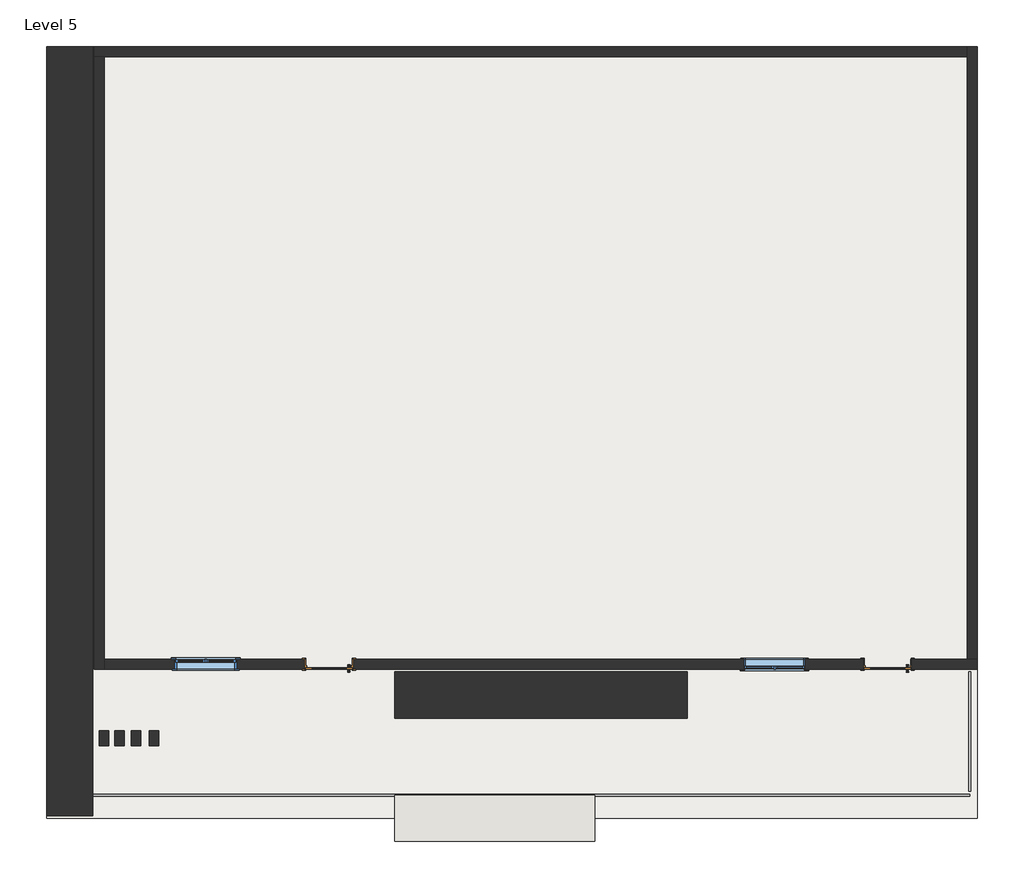
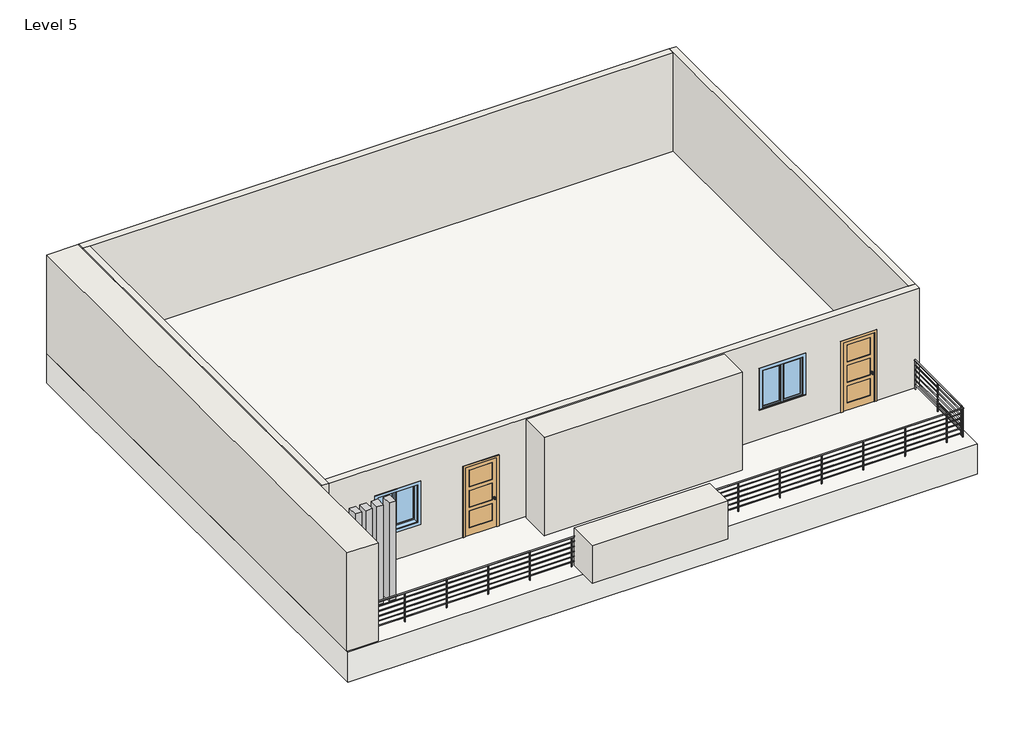
# One storey: 7 walls, 4 columns, 2 doors, 2 railings, 2 windows, 1 slab.
"""IFC4 building model written with IfcOpenShell, lengths in millimetres."""

from ifc_helpers import new_model, si_unit, point, frame, frame_2d, origin, place, context, project, spatial, polyline, circle_curve, trimmed, segment, composite_curve, outline, extrude, faceted_brep, transform, mapped, element, save
from components import wood_timber_column_8_x_12_7c9a4679, door_54d869bf, window_3a1167bf, window_0862ab64

model = new_model("IFC4")

# Units and contexts
model_context = context("Model", 3, world=origin())
ifc_project = project(units=[si_unit("LENGTHUNIT", "METRE", prefix="MILLI")], contexts=[model_context])

# Site, building, storey
site = spatial("IfcSite", under=ifc_project)
building = spatial("IfcBuilding", under=site)
storey = spatial("IfcBuildingStorey", under=building, Name="Level 5", Elevation=12192.0)

# Columns
placement = place(None, origin())
wood_timber_column_8_x_12_shape = wood_timber_column_8_x_12_7c9a4679(model_context)
element("IfcColumn", 1, ObjectType="Wood Timber Column : 8 x 12", at=placement, inside=storey, context=model_context, shape_type="MappedRepresentation", body=[
    mapped(wood_timber_column_8_x_12_shape, transform((-18270.7121948, 4590.8323495, 0.0), x_axis=(1.0, 0.0, 0.0), y_axis=(0.0, 1.0, 0.0), z_axis=(0.0, 0.0, 1.0))),
])
element("IfcColumn", 2, ObjectType="Wood Timber Column : 8 x 12", at=placement, inside=storey, context=model_context, shape_type="MappedRepresentation", body=[
    mapped(wood_timber_column_8_x_12_shape, transform((-18600.9121948, 4590.8323495, 0.0), x_axis=(1.0, 0.0, 0.0), y_axis=(0.0, 1.0, 0.0), z_axis=(0.0, 0.0, 1.0))),
])
element("IfcColumn", 3, ObjectType="Wood Timber Column : 8 x 12", at=placement, inside=storey, context=model_context, shape_type="MappedRepresentation", body=[
    mapped(wood_timber_column_8_x_12_shape, transform((-18905.7121948, 4590.8323495, 0.0), x_axis=(1.0, 0.0, 0.0), y_axis=(0.0, 1.0, 0.0), z_axis=(0.0, 0.0, 1.0))),
])
element("IfcColumn", 4, ObjectType="Wood Timber Column : 8 x 12", at=placement, inside=storey, context=model_context, shape_type="MappedRepresentation", body=[
    mapped(wood_timber_column_8_x_12_shape, transform((-17915.1121948, 4590.8323495, 0.0), x_axis=(1.0, 0.0, 0.0), y_axis=(0.0, 1.0, 0.0), z_axis=(0.0, 0.0, 1.0))),
])

# Doors
door_shape = door_54d869bf(model_context)
element("IfcDoor", 5, ObjectType="Door-Interior-Single-3_Panel_Vert-Wood : 36\" x 84\" 2", at=placement, inside=storey, context=model_context, shape_type="MappedRepresentation", body=[
    mapped(door_shape, transform((-3405.3621948, 6054.574368, 11845.2339631), x_axis=(-1.0, 0.0, 0.0), y_axis=(0.0, -1.0, 0.0), z_axis=(0.0, 0.0, 1.0))),
])
element("IfcDoor", 6, ObjectType="Door-Interior-Single-3_Panel_Vert-Wood : 36\" x 84\" 2", at=placement, inside=storey, context=model_context, shape_type="MappedRepresentation", body=[
    mapped(door_shape, transform((-14454.3621948, 6054.574368, 11845.2339631), x_axis=(-1.0, 0.0, 0.0), y_axis=(0.0, -1.0, 0.0), z_axis=(0.0, 0.0, 1.0))),
])

# Railings
element("IfcRailing", 7, ObjectType="Handrail - Pipe", at=placement, inside=storey, context=model_context, shape_type="SweptSolid", body=[
    extrude(outline(composite_curve([segment(trimmed(circle_curve(frame_2d((3466.949368, 12740.5839631)), 19.05), [point((3447.899368, 12740.5839631))], [point((3485.999368, 12740.5839631))], False, "CARTESIAN"), True, "CONTINUOUS"), segment(trimmed(circle_curve(frame_2d((3466.949368, 12740.5839631)), 19.05), [point((3485.999368, 12740.5839631))], [point((3447.899368, 12740.5839631))], False, "CARTESIAN"), True, "CONTINUOUS")], self_intersect=False)), frame((-19331.1621948, 0.0, 0.0), z_axis=(1.0, 0.0, 0.0), x_axis=(0.0, 1.0, 0.0)), (0.0, 0.0, 1.0), 17551.4),
    extrude(outline(composite_curve([segment(trimmed(circle_curve(frame_2d((3466.949368, 12594.5339631)), 12.7), [point((3479.649368, 12594.5339631))], [point((3454.249368, 12594.5339631))], False, "CARTESIAN"), True, "CONTINUOUS"), segment(trimmed(circle_curve(frame_2d((3466.949368, 12594.5339631)), 12.7), [point((3454.249368, 12594.5339631))], [point((3479.649368, 12594.5339631))], False, "CARTESIAN"), True, "CONTINUOUS")], self_intersect=False)), frame((-19331.1621948, 0.0, 0.0), z_axis=(1.0, 0.0, 0.0), x_axis=(0.0, 1.0, 0.0)), (0.0, 0.0, 1.0), 17551.4),
    extrude(outline(composite_curve([segment(trimmed(circle_curve(frame_2d((3466.949368, 12442.1339631)), 12.7), [point((3479.649368, 12442.1339631))], [point((3454.249368, 12442.1339631))], False, "CARTESIAN"), True, "CONTINUOUS"), segment(trimmed(circle_curve(frame_2d((3466.949368, 12442.1339631)), 12.7), [point((3454.249368, 12442.1339631))], [point((3479.649368, 12442.1339631))], False, "CARTESIAN"), True, "CONTINUOUS")], self_intersect=False)), frame((-19331.1621948, 0.0, 0.0), z_axis=(1.0, 0.0, 0.0), x_axis=(0.0, 1.0, 0.0)), (0.0, 0.0, 1.0), 17551.4),
    extrude(outline(composite_curve([segment(trimmed(circle_curve(frame_2d((3466.949368, 12289.7339631)), 12.7), [point((3479.649368, 12289.7339631))], [point((3454.249368, 12289.7339631))], False, "CARTESIAN"), True, "CONTINUOUS"), segment(trimmed(circle_curve(frame_2d((3466.949368, 12289.7339631)), 12.7), [point((3454.249368, 12289.7339631))], [point((3479.649368, 12289.7339631))], False, "CARTESIAN"), True, "CONTINUOUS")], self_intersect=False)), frame((-19331.1621948, 0.0, 0.0), z_axis=(1.0, 0.0, 0.0), x_axis=(0.0, 1.0, 0.0)), (0.0, 0.0, 1.0), 17551.4),
    extrude(outline(composite_curve([segment(trimmed(circle_curve(frame_2d((3466.949368, 12137.3339631)), 12.7), [point((3479.649368, 12137.3339631))], [point((3454.249368, 12137.3339631))], False, "CARTESIAN"), True, "CONTINUOUS"), segment(trimmed(circle_curve(frame_2d((3466.949368, 12137.3339631)), 12.7), [point((3454.249368, 12137.3339631))], [point((3479.649368, 12137.3339631))], False, "CARTESIAN"), True, "CONTINUOUS")], self_intersect=False)), frame((-19331.1621948, 0.0, 0.0), z_axis=(1.0, 0.0, 0.0), x_axis=(0.0, 1.0, 0.0)), (0.0, 0.0, 1.0), 17551.4),
    extrude(outline(composite_curve([segment(trimmed(circle_curve(frame_2d((3466.949368, 11984.9339631)), 12.7), [point((3479.649368, 11984.9339631))], [point((3454.249368, 11984.9339631))], False, "CARTESIAN"), True, "CONTINUOUS"), segment(trimmed(circle_curve(frame_2d((3466.949368, 11984.9339631)), 12.7), [point((3454.249368, 11984.9339631))], [point((3479.649368, 11984.9339631))], False, "CARTESIAN"), True, "CONTINUOUS")], self_intersect=False)), frame((-19331.1621948, 0.0, 0.0), z_axis=(1.0, 0.0, 0.0), x_axis=(0.0, 1.0, 0.0)), (0.0, 0.0, 1.0), 17551.4),
    extrude(outline(composite_curve([segment(trimmed(circle_curve(frame_2d((-2262.3621948, 3466.949368)), 12.7), [point((-2262.3621948, 3479.649368))], [point((-2262.3621948, 3454.249368))], False, "CARTESIAN"), True, "CONTINUOUS"), segment(trimmed(circle_curve(frame_2d((-2262.3621948, 3466.949368)), 12.7), [point((-2262.3621948, 3454.249368))], [point((-2262.3621948, 3479.649368))], False, "CARTESIAN"), True, "CONTINUOUS")], self_intersect=False)), frame((0.0, 0.0, 11845.2339631), z_axis=(0.0, 0.0, 1.0), x_axis=(1.0, 0.0, 0.0)), (0.0, 0.0, 1.0), 876.3),
    extrude(outline(composite_curve([segment(trimmed(circle_curve(frame_2d((-3481.5621948, 3466.949368)), 12.7), [point((-3481.5621948, 3479.649368))], [point((-3481.5621948, 3454.249368))], False, "CARTESIAN"), True, "CONTINUOUS"), segment(trimmed(circle_curve(frame_2d((-3481.5621948, 3466.949368)), 12.7), [point((-3481.5621948, 3454.249368))], [point((-3481.5621948, 3479.649368))], False, "CARTESIAN"), True, "CONTINUOUS")], self_intersect=False)), frame((0.0, 0.0, 11845.2339631), z_axis=(0.0, 0.0, 1.0), x_axis=(1.0, 0.0, 0.0)), (0.0, 0.0, 1.0), 876.3),
    extrude(outline(composite_curve([segment(trimmed(circle_curve(frame_2d((-4700.7621948, 3466.949368)), 12.7), [point((-4700.7621948, 3479.649368))], [point((-4700.7621948, 3454.249368))], False, "CARTESIAN"), True, "CONTINUOUS"), segment(trimmed(circle_curve(frame_2d((-4700.7621948, 3466.949368)), 12.7), [point((-4700.7621948, 3454.249368))], [point((-4700.7621948, 3479.649368))], False, "CARTESIAN"), True, "CONTINUOUS")], self_intersect=False)), frame((0.0, 0.0, 11845.2339631), z_axis=(0.0, 0.0, 1.0), x_axis=(1.0, 0.0, 0.0)), (0.0, 0.0, 1.0), 876.3),
    extrude(outline(composite_curve([segment(trimmed(circle_curve(frame_2d((-5919.9621948, 3466.949368)), 12.7), [point((-5919.9621948, 3479.649368))], [point((-5919.9621948, 3454.249368))], False, "CARTESIAN"), True, "CONTINUOUS"), segment(trimmed(circle_curve(frame_2d((-5919.9621948, 3466.949368)), 12.7), [point((-5919.9621948, 3454.249368))], [point((-5919.9621948, 3479.649368))], False, "CARTESIAN"), True, "CONTINUOUS")], self_intersect=False)), frame((0.0, 0.0, 11845.2339631), z_axis=(0.0, 0.0, 1.0), x_axis=(1.0, 0.0, 0.0)), (0.0, 0.0, 1.0), 876.3),
    extrude(outline(composite_curve([segment(trimmed(circle_curve(frame_2d((-7139.1621948, 3466.949368)), 12.7), [point((-7139.1621948, 3479.649368))], [point((-7139.1621948, 3454.249368))], False, "CARTESIAN"), True, "CONTINUOUS"), segment(trimmed(circle_curve(frame_2d((-7139.1621948, 3466.949368)), 12.7), [point((-7139.1621948, 3454.249368))], [point((-7139.1621948, 3479.649368))], False, "CARTESIAN"), True, "CONTINUOUS")], self_intersect=False)), frame((0.0, 0.0, 11845.2339631), z_axis=(0.0, 0.0, 1.0), x_axis=(1.0, 0.0, 0.0)), (0.0, 0.0, 1.0), 876.3),
    extrude(outline(composite_curve([segment(trimmed(circle_curve(frame_2d((-8358.3621948, 3466.949368)), 12.7), [point((-8358.3621948, 3479.649368))], [point((-8358.3621948, 3454.249368))], False, "CARTESIAN"), True, "CONTINUOUS"), segment(trimmed(circle_curve(frame_2d((-8358.3621948, 3466.949368)), 12.7), [point((-8358.3621948, 3454.249368))], [point((-8358.3621948, 3479.649368))], False, "CARTESIAN"), True, "CONTINUOUS")], self_intersect=False)), frame((0.0, 0.0, 11845.2339631), z_axis=(0.0, 0.0, 1.0), x_axis=(1.0, 0.0, 0.0)), (0.0, 0.0, 1.0), 876.3),
    extrude(outline(composite_curve([segment(trimmed(circle_curve(frame_2d((-9577.5621948, 3466.949368)), 12.7), [point((-9577.5621948, 3479.649368))], [point((-9577.5621948, 3454.249368))], False, "CARTESIAN"), True, "CONTINUOUS"), segment(trimmed(circle_curve(frame_2d((-9577.5621948, 3466.949368)), 12.7), [point((-9577.5621948, 3454.249368))], [point((-9577.5621948, 3479.649368))], False, "CARTESIAN"), True, "CONTINUOUS")], self_intersect=False)), frame((0.0, 0.0, 11845.2339631), z_axis=(0.0, 0.0, 1.0), x_axis=(1.0, 0.0, 0.0)), (0.0, 0.0, 1.0), 876.3),
    extrude(outline(composite_curve([segment(trimmed(circle_curve(frame_2d((-10796.7621948, 3466.949368)), 12.7), [point((-10796.7621948, 3479.649368))], [point((-10796.7621948, 3454.249368))], False, "CARTESIAN"), True, "CONTINUOUS"), segment(trimmed(circle_curve(frame_2d((-10796.7621948, 3466.949368)), 12.7), [point((-10796.7621948, 3454.249368))], [point((-10796.7621948, 3479.649368))], False, "CARTESIAN"), True, "CONTINUOUS")], self_intersect=False)), frame((0.0, 0.0, 11845.2339631), z_axis=(0.0, 0.0, 1.0), x_axis=(1.0, 0.0, 0.0)), (0.0, 0.0, 1.0), 876.3),
    extrude(outline(composite_curve([segment(trimmed(circle_curve(frame_2d((-12015.9621948, 3466.949368)), 12.7), [point((-12015.9621948, 3479.649368))], [point((-12015.9621948, 3454.249368))], False, "CARTESIAN"), True, "CONTINUOUS"), segment(trimmed(circle_curve(frame_2d((-12015.9621948, 3466.949368)), 12.7), [point((-12015.9621948, 3454.249368))], [point((-12015.9621948, 3479.649368))], False, "CARTESIAN"), True, "CONTINUOUS")], self_intersect=False)), frame((0.0, 0.0, 11845.2339631), z_axis=(0.0, 0.0, 1.0), x_axis=(1.0, 0.0, 0.0)), (0.0, 0.0, 1.0), 876.3),
    extrude(outline(composite_curve([segment(trimmed(circle_curve(frame_2d((-13235.1621948, 3466.949368)), 12.7), [point((-13235.1621948, 3479.649368))], [point((-13235.1621948, 3454.249368))], False, "CARTESIAN"), True, "CONTINUOUS"), segment(trimmed(circle_curve(frame_2d((-13235.1621948, 3466.949368)), 12.7), [point((-13235.1621948, 3454.249368))], [point((-13235.1621948, 3479.649368))], False, "CARTESIAN"), True, "CONTINUOUS")], self_intersect=False)), frame((0.0, 0.0, 11845.2339631), z_axis=(0.0, 0.0, 1.0), x_axis=(1.0, 0.0, 0.0)), (0.0, 0.0, 1.0), 876.3),
    extrude(outline(composite_curve([segment(trimmed(circle_curve(frame_2d((-14454.3621948, 3466.949368)), 12.7), [point((-14454.3621948, 3479.649368))], [point((-14454.3621948, 3454.249368))], False, "CARTESIAN"), True, "CONTINUOUS"), segment(trimmed(circle_curve(frame_2d((-14454.3621948, 3466.949368)), 12.7), [point((-14454.3621948, 3454.249368))], [point((-14454.3621948, 3479.649368))], False, "CARTESIAN"), True, "CONTINUOUS")], self_intersect=False)), frame((0.0, 0.0, 11845.2339631), z_axis=(0.0, 0.0, 1.0), x_axis=(1.0, 0.0, 0.0)), (0.0, 0.0, 1.0), 876.3),
    extrude(outline(composite_curve([segment(trimmed(circle_curve(frame_2d((-15673.5621948, 3466.949368)), 12.7), [point((-15673.5621948, 3479.649368))], [point((-15673.5621948, 3454.249368))], False, "CARTESIAN"), True, "CONTINUOUS"), segment(trimmed(circle_curve(frame_2d((-15673.5621948, 3466.949368)), 12.7), [point((-15673.5621948, 3454.249368))], [point((-15673.5621948, 3479.649368))], False, "CARTESIAN"), True, "CONTINUOUS")], self_intersect=False)), frame((0.0, 0.0, 11845.2339631), z_axis=(0.0, 0.0, 1.0), x_axis=(1.0, 0.0, 0.0)), (0.0, 0.0, 1.0), 876.3),
    extrude(outline(composite_curve([segment(trimmed(circle_curve(frame_2d((-16892.7621948, 3466.949368)), 12.7), [point((-16892.7621948, 3479.649368))], [point((-16892.7621948, 3454.249368))], False, "CARTESIAN"), True, "CONTINUOUS"), segment(trimmed(circle_curve(frame_2d((-16892.7621948, 3466.949368)), 12.7), [point((-16892.7621948, 3454.249368))], [point((-16892.7621948, 3479.649368))], False, "CARTESIAN"), True, "CONTINUOUS")], self_intersect=False)), frame((0.0, 0.0, 11845.2339631), z_axis=(0.0, 0.0, 1.0), x_axis=(1.0, 0.0, 0.0)), (0.0, 0.0, 1.0), 876.3),
    extrude(outline(composite_curve([segment(trimmed(circle_curve(frame_2d((-18111.9621948, 3466.949368)), 12.7), [point((-18111.9621948, 3479.649368))], [point((-18111.9621948, 3454.249368))], False, "CARTESIAN"), True, "CONTINUOUS"), segment(trimmed(circle_curve(frame_2d((-18111.9621948, 3466.949368)), 12.7), [point((-18111.9621948, 3454.249368))], [point((-18111.9621948, 3479.649368))], False, "CARTESIAN"), True, "CONTINUOUS")], self_intersect=False)), frame((0.0, 0.0, 11845.2339631), z_axis=(0.0, 0.0, 1.0), x_axis=(1.0, 0.0, 0.0)), (0.0, 0.0, 1.0), 876.3),
    extrude(outline(composite_curve([segment(trimmed(circle_curve(frame_2d((-1792.4621948, 3466.949368)), 12.7), [point((-1792.4621948, 3479.649368))], [point((-1792.4621948, 3454.249368))], False, "CARTESIAN"), True, "CONTINUOUS"), segment(trimmed(circle_curve(frame_2d((-1792.4621948, 3466.949368)), 12.7), [point((-1792.4621948, 3454.249368))], [point((-1792.4621948, 3479.649368))], False, "CARTESIAN"), True, "CONTINUOUS")], self_intersect=False)), frame((0.0, 0.0, 11845.2339631), z_axis=(0.0, 0.0, 1.0), x_axis=(1.0, 0.0, 0.0)), (0.0, 0.0, 1.0), 876.3),
    extrude(outline(composite_curve([segment(trimmed(circle_curve(frame_2d((-19318.4621948, 3466.949368)), 12.7), [point((-19318.4621948, 3479.649368))], [point((-19318.4621948, 3454.249368))], False, "CARTESIAN"), True, "CONTINUOUS"), segment(trimmed(circle_curve(frame_2d((-19318.4621948, 3466.949368)), 12.7), [point((-19318.4621948, 3454.249368))], [point((-19318.4621948, 3479.649368))], False, "CARTESIAN"), True, "CONTINUOUS")], self_intersect=False)), frame((0.0, 0.0, 11845.2339631), z_axis=(0.0, 0.0, 1.0), x_axis=(1.0, 0.0, 0.0)), (0.0, 0.0, 1.0), 876.3),
])
element("IfcRailing", 8, ObjectType="Handrail - Pipe", at=placement, inside=storey, context=model_context, shape_type="SweptSolid", body=[
    extrude(outline(composite_curve([segment(trimmed(circle_curve(frame_2d((12740.5839631, -1779.7621948)), 19.05), [point((12740.5839631, -1760.7121948))], [point((12740.5839631, -1798.8121948))], False, "CARTESIAN"), True, "CONTINUOUS"), segment(trimmed(circle_curve(frame_2d((12740.5839631, -1779.7621948)), 19.05), [point((12740.5839631, -1798.8121948))], [point((12740.5839631, -1760.7121948))], False, "CARTESIAN"), True, "CONTINUOUS")], self_intersect=False)), frame((0.0, 3543.149368, 0.0), z_axis=(0.0, 1.0, 0.0), x_axis=(0.0, 0.0, 1.0)), (0.0, 0.0, 1.0), 2362.2),
    extrude(outline(composite_curve([segment(trimmed(circle_curve(frame_2d((12594.5339631, -1779.7621948)), 12.7), [point((12594.5339631, -1792.4621948))], [point((12594.5339631, -1767.0621948))], False, "CARTESIAN"), True, "CONTINUOUS"), segment(trimmed(circle_curve(frame_2d((12594.5339631, -1779.7621948)), 12.7), [point((12594.5339631, -1767.0621948))], [point((12594.5339631, -1792.4621948))], False, "CARTESIAN"), True, "CONTINUOUS")], self_intersect=False)), frame((0.0, 3543.149368, 0.0), z_axis=(0.0, 1.0, 0.0), x_axis=(0.0, 0.0, 1.0)), (0.0, 0.0, 1.0), 2362.2),
    extrude(outline(composite_curve([segment(trimmed(circle_curve(frame_2d((12442.1339631, -1779.7621948)), 12.7), [point((12442.1339631, -1792.4621948))], [point((12442.1339631, -1767.0621948))], False, "CARTESIAN"), True, "CONTINUOUS"), segment(trimmed(circle_curve(frame_2d((12442.1339631, -1779.7621948)), 12.7), [point((12442.1339631, -1767.0621948))], [point((12442.1339631, -1792.4621948))], False, "CARTESIAN"), True, "CONTINUOUS")], self_intersect=False)), frame((0.0, 3543.149368, 0.0), z_axis=(0.0, 1.0, 0.0), x_axis=(0.0, 0.0, 1.0)), (0.0, 0.0, 1.0), 2362.2),
    extrude(outline(composite_curve([segment(trimmed(circle_curve(frame_2d((12289.7339631, -1779.7621948)), 12.7), [point((12289.7339631, -1792.4621948))], [point((12289.7339631, -1767.0621948))], False, "CARTESIAN"), True, "CONTINUOUS"), segment(trimmed(circle_curve(frame_2d((12289.7339631, -1779.7621948)), 12.7), [point((12289.7339631, -1767.0621948))], [point((12289.7339631, -1792.4621948))], False, "CARTESIAN"), True, "CONTINUOUS")], self_intersect=False)), frame((0.0, 3543.149368, 0.0), z_axis=(0.0, 1.0, 0.0), x_axis=(0.0, 0.0, 1.0)), (0.0, 0.0, 1.0), 2362.2),
    extrude(outline(composite_curve([segment(trimmed(circle_curve(frame_2d((12137.3339631, -1779.7621948)), 12.7), [point((12137.3339631, -1792.4621948))], [point((12137.3339631, -1767.0621948))], False, "CARTESIAN"), True, "CONTINUOUS"), segment(trimmed(circle_curve(frame_2d((12137.3339631, -1779.7621948)), 12.7), [point((12137.3339631, -1767.0621948))], [point((12137.3339631, -1792.4621948))], False, "CARTESIAN"), True, "CONTINUOUS")], self_intersect=False)), frame((0.0, 3543.149368, 0.0), z_axis=(0.0, 1.0, 0.0), x_axis=(0.0, 0.0, 1.0)), (0.0, 0.0, 1.0), 2362.2),
    extrude(outline(composite_curve([segment(trimmed(circle_curve(frame_2d((11984.9339631, -1779.7621948)), 12.7), [point((11984.9339631, -1792.4621948))], [point((11984.9339631, -1767.0621948))], False, "CARTESIAN"), True, "CONTINUOUS"), segment(trimmed(circle_curve(frame_2d((11984.9339631, -1779.7621948)), 12.7), [point((11984.9339631, -1767.0621948))], [point((11984.9339631, -1792.4621948))], False, "CARTESIAN"), True, "CONTINUOUS")], self_intersect=False)), frame((0.0, 3543.149368, 0.0), z_axis=(0.0, 1.0, 0.0), x_axis=(0.0, 0.0, 1.0)), (0.0, 0.0, 1.0), 2362.2),
    extrude(outline(composite_curve([segment(trimmed(circle_curve(frame_2d((-1779.7621948, 4762.349368)), 12.7), [point((-1792.4621948, 4762.349368))], [point((-1767.0621948, 4762.349368))], False, "CARTESIAN"), True, "CONTINUOUS"), segment(trimmed(circle_curve(frame_2d((-1779.7621948, 4762.349368)), 12.7), [point((-1767.0621948, 4762.349368))], [point((-1792.4621948, 4762.349368))], False, "CARTESIAN"), True, "CONTINUOUS")], self_intersect=False)), frame((0.0, 0.0, 11845.2339631), z_axis=(0.0, 0.0, 1.0), x_axis=(1.0, 0.0, 0.0)), (0.0, 0.0, 1.0), 876.3),
    extrude(outline(composite_curve([segment(trimmed(circle_curve(frame_2d((-1779.7621948, 5892.649368)), 12.7), [point((-1792.4621948, 5892.649368))], [point((-1767.0621948, 5892.649368))], False, "CARTESIAN"), True, "CONTINUOUS"), segment(trimmed(circle_curve(frame_2d((-1779.7621948, 5892.649368)), 12.7), [point((-1767.0621948, 5892.649368))], [point((-1792.4621948, 5892.649368))], False, "CARTESIAN"), True, "CONTINUOUS")], self_intersect=False)), frame((0.0, 0.0, 11845.2339631), z_axis=(0.0, 0.0, 1.0), x_axis=(1.0, 0.0, 0.0)), (0.0, 0.0, 1.0), 876.3),
    extrude(outline(composite_curve([segment(trimmed(circle_curve(frame_2d((-1779.7621948, 3555.849368)), 12.7), [point((-1792.4621948, 3555.849368))], [point((-1767.0621948, 3555.849368))], False, "CARTESIAN"), True, "CONTINUOUS"), segment(trimmed(circle_curve(frame_2d((-1779.7621948, 3555.849368)), 12.7), [point((-1767.0621948, 3555.849368))], [point((-1792.4621948, 3555.849368))], False, "CARTESIAN"), True, "CONTINUOUS")], self_intersect=False)), frame((0.0, 0.0, 11845.2339631), z_axis=(0.0, 0.0, 1.0), x_axis=(1.0, 0.0, 0.0)), (0.0, 0.0, 1.0), 876.3),
])

# Slab
element("IfcSlab", 9, ObjectType="Generic - 3'", at=placement, inside=storey, context=model_context, shape_type="SweptSolid", body=[
    extrude(outline(polyline([(-1627.3621948, 18275.149368), (-1627.3621948, 3009.749368), (-20042.3621948, 3009.749368), (-20042.3621948, 18275.149368), (-1627.3621948, 18275.149368)])), frame((0.0, 0.0, 10930.8339631), z_axis=(0.0, 0.0, 1.0), x_axis=(1.0, 0.0, 0.0)), (0.0, 0.0, 1.0), 914.4),
])

# Walls
element("IfcWall", 10, ObjectType="Generic - 3' 2", at=placement, inside=storey, context=model_context, shape_type="SweptSolid", body=[
    extrude(outline(polyline([(-7367.7621948, 4990.949368), (-13158.9621948, 4990.949368), (-13158.9621948, 5905.349368), (-7367.7621948, 5905.349368), (-7367.7621948, 4990.949368)])), frame((0.0, 0.0, 11845.2339631), z_axis=(0.0, 0.0, 1.0), x_axis=(1.0, 0.0, 0.0)), (0.0, 0.0, 1.0), 3048.0),
])
element("IfcWall", 11, ObjectType="Generic - 3' 4", at=placement, inside=storey, context=model_context, shape_type="SweptSolid", body=[
    extrude(outline(polyline([(-9196.5621948, 2552.549368), (-13158.9621948, 2552.549368), (-13158.9621948, 3466.949368), (-9196.5621948, 3466.949368), (-9196.5621948, 2552.549368)])), frame((0.0, 0.0, 11845.2339631), z_axis=(0.0, 0.0, 1.0), x_axis=(1.0, 0.0, 0.0)), (0.0, 0.0, 1.0), 1165.3811612),
])
element("IfcWall", 12, ObjectType="Generic - 3' 4", at=placement, inside=storey, context=model_context, shape_type="SweptSolid", body=[
    extrude(outline(polyline([(-20042.3621948, 3060.549368), (-20042.3621948, 18275.149368), (-19127.9621948, 18275.149368), (-19127.9621948, 3060.549368), (-20042.3621948, 3060.549368)])), frame((0.0, 0.0, 11845.2339631), z_axis=(0.0, 0.0, 1.0), x_axis=(1.0, 0.0, 0.0)), (0.0, 0.0, 1.0), 3048.0),
])
element("IfcWall", 13, ObjectType="Generic - 8\"", at=placement, inside=storey, context=model_context, shape_type="Brep", body=[
    faceted_brep([(-19102.5621948, 18071.949368, 11845.2339631), (-18899.3621948, 18071.949368, 11845.2339631), (-1830.5621948, 18071.949368, 11845.2339631), (-1830.5621948, 18071.949368, 14893.2339631), (-18899.3621948, 18071.949368, 14893.2339631), (-19102.5621948, 18071.949368, 14893.2339631), (-19102.5621948, 18275.149368, 11845.2339631), (-19102.5621948, 18275.149368, 14893.2339631), (-1830.5621948, 18275.149368, 14893.2339631), (-1830.5621948, 18275.149368, 11845.2339631)], [[[0, 1, 2, 3, 4, 5]], [[6, 7, 8, 9]], [[2, 1, 0, 6, 9]], [[5, 4, 3, 8, 7]], [[0, 5, 7, 6]], [[3, 2, 9, 8]]]),
])
element("IfcWall", 14, ObjectType="Generic - 8\"", at=placement, inside=storey, context=model_context, shape_type="Brep", body=[
    faceted_brep([(-18899.3621948, 6159.349368, 14893.2339631), (-1830.5621948, 6159.349368, 14893.2339631), (-1627.3621948, 6159.349368, 14893.2339631), (-1627.3621948, 6159.349368, 11845.2339631), (-1830.5621948, 6159.349368, 11845.2339631), (-2922.7621948, 6159.349368, 11845.2339631), (-2922.7621948, 6159.349368, 14004.2339631), (-3887.9621948, 6159.349368, 14004.2339631), (-3887.9621948, 6159.349368, 11845.2339631), (-13971.7621948, 6159.349368, 11845.2339631), (-13971.7621948, 6159.349368, 14004.2339631), (-14936.9621948, 6159.349368, 14004.2339631), (-14936.9621948, 6159.349368, 11845.2339631), (-18899.3621948, 6159.349368, 11845.2339631), (-17502.3621948, 6159.349368, 13978.8339631), (-17502.3621948, 6159.349368, 12759.6339631), (-16283.1621948, 6159.349368, 12759.6339631), (-16283.1621948, 6159.349368, 13978.8339631), (-6250.1621948, 6159.349368, 13978.8339631), (-6250.1621948, 6159.349368, 12759.6339631), (-5030.9621948, 6159.349368, 12759.6339631), (-5030.9621948, 6159.349368, 13978.8339631), (-1627.3621948, 5956.149368, 14893.2339631), (-18899.3621948, 5956.149368, 14893.2339631), (-18899.3621948, 5956.149368, 11845.2339631), (-14936.9621948, 5956.149368, 11845.2339631), (-14936.9621948, 5956.149368, 14004.2339631), (-13971.7621948, 5956.149368, 14004.2339631), (-13971.7621948, 5956.149368, 11845.2339631), (-3887.9621948, 5956.149368, 11845.2339631), (-3887.9621948, 5956.149368, 14004.2339631), (-2922.7621948, 5956.149368, 14004.2339631), (-2922.7621948, 5956.149368, 11845.2339631), (-1627.3621948, 5956.149368, 11845.2339631), (-17502.3621948, 5956.149368, 13978.8339631), (-16283.1621948, 5956.149368, 13978.8339631), (-16283.1621948, 5956.149368, 12759.6339631), (-17502.3621948, 5956.149368, 12759.6339631), (-6250.1621948, 5956.149368, 13978.8339631), (-5030.9621948, 5956.149368, 13978.8339631), (-5030.9621948, 5956.149368, 12759.6339631), (-6250.1621948, 5956.149368, 12759.6339631)], [[[0, 1, 2, 3, 4, 5, 6, 7, 8, 9, 10, 11, 12, 13], [14, 15, 16, 17], [18, 19, 20, 21]], [[22, 23, 24, 25, 26, 27, 28, 29, 30, 31, 32, 33], [34, 35, 36, 37], [38, 39, 40, 41]], [[3, 33, 32, 5, 4]], [[8, 29, 28, 9]], [[24, 13, 12, 25]], [[2, 1, 0, 23, 22]], [[3, 2, 22, 33]], [[7, 30, 29, 8]], [[30, 7, 6, 31]], [[31, 6, 5, 32]], [[11, 26, 25, 12]], [[26, 11, 10, 27]], [[27, 10, 9, 28]], [[15, 14, 34, 37]], [[16, 15, 37, 36]], [[17, 16, 36, 35]], [[14, 17, 35, 34]], [[19, 18, 38, 41]], [[20, 19, 41, 40]], [[21, 20, 40, 39]], [[18, 21, 39, 38]], [[0, 13, 24, 23]]]),
])
element("IfcWall", 15, ObjectType="Generic - 8\"", at=placement, inside=storey, context=model_context, shape_type="Brep", body=[
    faceted_brep([(-1830.5621948, 18275.149368, 11845.2339631), (-1830.5621948, 18071.949368, 11845.2339631), (-1830.5621948, 6159.349368, 11845.2339631), (-1830.5621948, 6159.349368, 14893.2339631), (-1830.5621948, 18071.949368, 14893.2339631), (-1830.5621948, 18275.149368, 14893.2339631), (-1627.3621948, 18275.149368, 11845.2339631), (-1627.3621948, 18275.149368, 14893.2339631), (-1627.3621948, 6159.349368, 14893.2339631), (-1627.3621948, 6159.349368, 11845.2339631)], [[[0, 1, 2, 3, 4, 5]], [[6, 7, 8, 9]], [[2, 1, 0, 6, 9]], [[5, 4, 3, 8, 7]], [[0, 5, 7, 6]], [[3, 2, 9, 8]]]),
])
element("IfcWall", 16, ObjectType="Generic - 8\"", at=placement, inside=storey, context=model_context, shape_type="Brep", body=[
    faceted_brep([(-18899.3621948, 5956.149368, 11845.2339631), (-18899.3621948, 6159.349368, 11845.2339631), (-18899.3621948, 18071.949368, 11845.2339631), (-18899.3621948, 18071.949368, 14893.2339631), (-18899.3621948, 6159.349368, 14893.2339631), (-18899.3621948, 5956.149368, 14893.2339631), (-19102.5621948, 5956.149368, 11845.2339631), (-19102.5621948, 5956.149368, 14893.2339631), (-19102.5621948, 18071.949368, 14893.2339631), (-19102.5621948, 18071.949368, 11845.2339631)], [[[0, 1, 2, 3, 4, 5]], [[6, 7, 8, 9]], [[2, 1, 0, 6, 9]], [[5, 4, 3, 8, 7]], [[3, 2, 9, 8]], [[0, 5, 7, 6]]]),
])

# Windows
window_shape = window_3a1167bf(model_context)
element("IfcWindow", 17, ObjectType="Casement Dbl with Trim : 48\" x 48\"", at=placement, inside=storey, context=model_context, shape_type="MappedRepresentation", body=[
    mapped(window_shape, transform((-16892.7621948, 6038.699368, 11845.2339631), x_axis=(-1.0, 0.0, 0.0), y_axis=(0.0, -1.0, 0.0), z_axis=(0.0, 0.0, 1.0))),
])
window_2_shape = window_0862ab64(model_context)
element("IfcWindow", 18, ObjectType="Casement Dbl with Trim : 48\" x 48\" 2", at=placement, inside=storey, context=model_context, shape_type="MappedRepresentation", body=[
    mapped(window_2_shape, transform((-5640.5621948, 6076.799368, 11845.2339631), x_axis=(-1.0, 0.0, 0.0), y_axis=(0.0, -1.0, 0.0), z_axis=(0.0, 0.0, 1.0))),
])

save(model, "model.ifc")

# Revit data of these elements
# Type "Wood Timber Column : 8 x 12"
#   Assembly Code = "B1010200"
#   Depth = 0' - 11 1/2"
#   Width = 0' - 7 1/2"
#   Material = Softwood, Lumber
# Type "Door-Interior-Single-3_Panel_Vert-Wood : 36\" x 84\" 2"
#   Type Mark = "11"
#   Assembly Code = "C1020300"
#   Analytic Construction = "Wooden"
#   Top Rail = 0' - 4 11/16"
#   Thickness = 0' - 1 3/8"
#   Thermal Resistance (R) = 2.5876 (h·ft²·°F)/BTU
#   Swing Angle [instance default] = 90.00°
#   Stiles = 0' - 4 3/4"
#   Rough Width = 3' - 2"
#   Rough Height = 7' - 1"
#   Intermediate Rail = 0' - 4 1/2"
#   Height = 7' - 0"
#   Width = 3' - 0"
#   Heat Transfer Coefficient (U) = 0.3865 BTU/(h·ft²·°F)
#   Bottom Rail = 0' - 9 1/8"
#   Trim Material = Cherry
#   Panel Material = Door - Panel
#   Frame Material = Door - Panel
#   Door Handle Material = Aluminum
#   Visual Light Transmittance = 0
#   Solar Heat Gain Coefficient = 0
#   Wall Closure = (empty or 0)
#   Function = (empty or 0)
# Type "Handrail - Pipe"
#   Assembly Code = "C2010400"
#   built-in parameter 1008612 = 0.0416667 (stored number, unit not read)
#   built-in parameter 1008611 = 0.0833333 (stored number, unit not read)
#   built-in parameter 1008609 = 4 (stored number, unit not read)
#   built-in parameter 1008604 = 0.166667 (stored number, unit not read)
#   built-in parameter 1008603 = 0.166667 (stored number, unit not read)
#   Railing Height = 3' - 0"
#   built-in parameter 1008630 = 2
#   built-in parameter 1008610 = 1
#   built-in parameter 1008605 = 1
#   built-in parameter 1008618 = Baluster - Round : 1"
# Type "Generic - 3'"
#   Assembly Code = "B1010"
#   Function = 0
#   Layers, outside or top first: 3' - 0" "Parking Stripe" (function 1)
# Type "Generic - 3' 2"
#   Assembly Code = "B2010"
#   Layers, outside or top first: 3' - 0" "Asphalt Shingle" (function 1)
# Type "Generic - 3' 4"
#   Assembly Code = "B2010"
#   Layers, outside or top first: 3' - 0" "Parking Stripe" (function 1)
# Type "Generic - 8\""
#   Assembly Code = "B2010"
#   Layers, outside or top first: 0' - 8" "Paint - Sienna" (function 1)
# Type "Casement Dbl with Trim : 48\" x 48\""
#   Type Mark = "10"
#   Construction Type Id = "GSP4R"
#   Assembly Code = "B2020100"
#   Analytic Construction = "1/8 in Pilkington single glazing"
#   Visual Light Transmittance = 0.9
#   Thermal Resistance (R) = 1.53941 (h·ft²·°F)/BTU
#   Solar Heat Gain Coefficient = 0.78
#   Heat Transfer Coefficient (U) = 0.6496 BTU/(h·ft²·°F)
#   Height = 4' - 0"
#   Default Sill Height = 3' - 0"
#   Trim Projection - Ext. = 0' - 0 1/2"
#   Trim Projection - Int. = 0' - 0 3/4"
#   Trim Width - Exterior = 0' - 3 1/2"
#   Trim Width - Interior = 0' - 3 1/2"
#   Width = 4' - 0"
#   Window Inset = 0' - 0 3/4"
#   Define Thermal Properties by = 1
#   Glass Pane Material = Glass
#   Sash Material = Sash
#   Trim Exterior Material = Trim
#   Trim Interior Material = Trim
#   Wall Closure = (empty or 0)
# Type "Casement Dbl with Trim : 48\" x 48\" 2"
#   Type Mark = "13"
#   Construction Type Id = "GSP4R"
#   Assembly Code = "B2020100"
#   Analytic Construction = "1/8 in Pilkington single glazing"
#   Visual Light Transmittance = 0.9
#   Thermal Resistance (R) = 1.53941 (h·ft²·°F)/BTU
#   Solar Heat Gain Coefficient = 0.78
#   Heat Transfer Coefficient (U) = 0.6496 BTU/(h·ft²·°F)
#   Height = 4' - 0"
#   Default Sill Height = 3' - 0"
#   Trim Projection - Ext. = 0' - 0 1/2"
#   Trim Projection - Int. = 0' - 0 3/4"
#   Trim Width - Exterior = 0' - 3 1/2"
#   Trim Width - Interior = 0' - 3 1/2"
#   Width = 4' - 0"
#   Window Inset = 0' - 0 3/4"
#   Define Thermal Properties by = 1
#   Glass Pane Material = Glass, Clear Glazing
#   Sash Material = Copper
#   Trim Exterior Material = Earth
#   Trim Interior Material = Earth
#   Wall Closure = (empty or 0)
# Elements 1, 2, 3, 4 (IfcColumn, "Wood Timber Column : 8 x 12")
#   Phase Created = New Construction
#   Materials on its faces: "Softwood, Lumber"
# Elements 5, 6 (IfcDoor, "Door-Interior-Single-3_Panel_Vert-Wood : 36\" x 84\" 2")
#   Swing Angle = 90.00°
#   Phase Created = New Construction
#   Materials on its faces: "Door - Panel", "Aluminum", "Cherry"
# Elements 7, 8 (IfcRailing, "Handrail - Pipe")
#   built-in parameter 1008621 = -1.13768 (stored number, unit not read)
#   Phase Created = New Construction
# Element 9 (IfcSlab, "Generic - 3'")
#   Height Offset From Level = -1' - 1.65221"
#   Phase Created = New Construction
#   Materials on its faces: "Parking Stripe"
# Element 10 (IfcWall, "Generic - 3' 2")
#   built-in parameter 1001111 = -1' - 1.65221"
#   Top Offset = 0' - 0"
#   Base Offset = -1' - 1.65221"
#   Unconnected Height = 10' - 0"
#   wall height = 10' - 0"
#   Phase Created = New Construction
#   Base Constraint = Level 5
#   Materials on its faces: "Asphalt Shingle"
# Element 11 (IfcWall, "Generic - 3' 4")
#   built-in parameter 1001111 = -1' - 1.65221"
#   Top Offset = 0' - 0"
#   Base Offset = -1' - 1.65221"
#   Unconnected Height = 3' - 9.88115"
#   wall height = 3' - 9.88115"
#   Phase Created = New Construction
#   Base Constraint = Level 5
#   Materials on its faces: "Parking Stripe"
# Element 12 (IfcWall, "Generic - 3' 4")
#   built-in parameter 1001111 = -1' - 1.65221"
#   Top Offset = 0' - 0"
#   Base Offset = -1' - 1.65221"
#   Unconnected Height = 10' - 0"
#   wall height = 10' - 0"
#   Phase Created = New Construction
#   Base Constraint = Level 5
#   Materials on its faces: "Parking Stripe"
# Elements 13, 14, 15, 16 (IfcWall, "Generic - 8\"")
#   built-in parameter 1001111 = -1' - 1.65221"
#   Top Offset = 0' - 0"
#   Base Offset = -1' - 1.65221"
#   Unconnected Height = 10' - 0"
#   wall height = 10' - 0"
#   Phase Created = New Construction
#   Base Constraint = Level 5
#   Materials on its faces: "Paint - Sienna"
# Element 17 (IfcWindow, "Casement Dbl with Trim : 48\" x 48\"")
#   Mark = "10"
#   Phase Created = New Construction
#   Materials on its faces: "Sash", "Trim", "Glass"
# Element 18 (IfcWindow, "Casement Dbl with Trim : 48\" x 48\" 2")
#   Mark = "11"
#   Phase Created = New Construction
#   Materials on its faces: "Copper", "Earth", "Glass, Clear Glazing"
# Materials
#   "Softwood, Lumber": class "Wood", colour RGB 223 192 134, transparency 0, Description = "Pinus Echinata", Cost = 0
#   "Cherry": class "Wood", colour RGB 226 177 128, transparency 0, Description = "Prunus Serotina", Cost = 0
#   "Door - Panel": class "Wood", colour RGB 210 159 95, transparency 0
#   "Aluminum": class "Metal", colour RGB 247 247 247, transparency 0, Description = "Aluminum 6061", Cost = 0
#   "Parking Stripe": class "Paint", colour RGB 255 221 187, transparency 0, Cost = 0
#   "Asphalt Shingle": class "Generic", colour RGB 155 155 155, transparency 0, Description = "Asphalt roofing shingle", Cost = 0
#   "Paint - Sienna": colour RGB 255 255 255, transparency 0, Cost = 0
#   "Glass": class "Glass", colour RGB 0 128 192, transparency 0.75, Description = "Soda Lime Glass", Cost = 0
#   "Sash": class "Wood", colour RGB 224 178 126, transparency 0
#   "Trim": class "Wood", colour RGB 224 178 126, transparency 0
#   "Glass, Clear Glazing": class "Glass", colour RGB 0 128 192, transparency 0.75, Description = "Clear glazing", Cost = 0
#   "Copper": class "Metal", colour RGB 0 0 0, transparency 0, Description = "Copper, matte finish", Cost = 0
#   "Earth": class "Generic", colour RGB 97 75 62, transparency 0, Description = "Soil", Cost = 0
